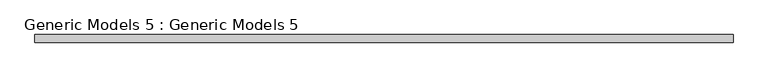
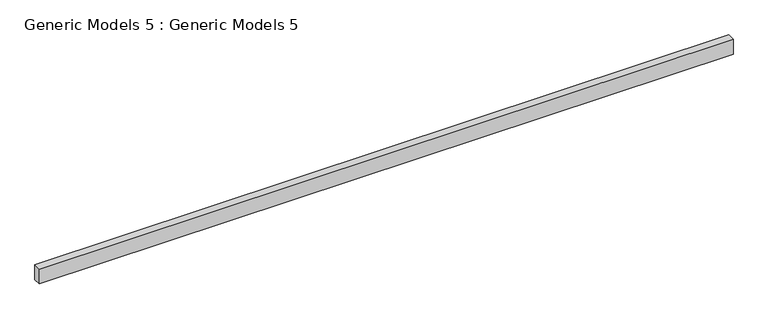
"""IFC4 building model written with IfcOpenShell, lengths in millimetres: proxy geometry, Generic Models 5 : Generic Models 5."""

from ifc_helpers import new_model, si_unit, frame, origin, place, context, project, spatial, polyline, outline, extrude, source, transform, mapped, element, save


def generic_models_5_generic_models_5_c0e4cdeb(model_context):
    return source(origin(), model_context, "Body", "SweptSolid", [
        extrude(outline(polyline([(12501.479405, -3746.0004242), (12501.479405, -3980.909008), (-8934.7629849, -3980.909008), (-8934.7629849, -3746.0004242), (12501.479405, -3746.0004242)])), frame((0.0, 0.0, 9416.8101851), z_axis=(0.0, 0.0, 1.0), x_axis=(1.0, 0.0, 0.0)), (0.0, 0.0, 1.0), 489.1898149),
    ])


if __name__ == "__main__":
    model = new_model("IFC4")
    model_context = context("Model", 3, world=origin())
    ifc_project = project(units=[si_unit("LENGTHUNIT", "METRE", prefix="MILLI")], contexts=[model_context])
    site = spatial("IfcSite", under=ifc_project)
    building = spatial("IfcBuilding", under=site)
    placement = place(None, origin())
    generic_models_5_generic_models_5_shape = generic_models_5_generic_models_5_c0e4cdeb(model_context)
    element("IfcBuildingElementProxy", 1, Name="Generic Models 5 : Generic Models 5", ObjectType="Generic Models 5 : Generic Models 5", at=placement, inside=building, context=model_context, shape_type="MappedRepresentation", body=[
        mapped(generic_models_5_generic_models_5_shape, transform((0.0, 0.0, 0.0), x_axis=(1.0, 0.0, 0.0), y_axis=(0.0, 1.0, 0.0), z_axis=(0.0, 0.0, 1.0))),
    ])
    save(model, "model.ifc")
